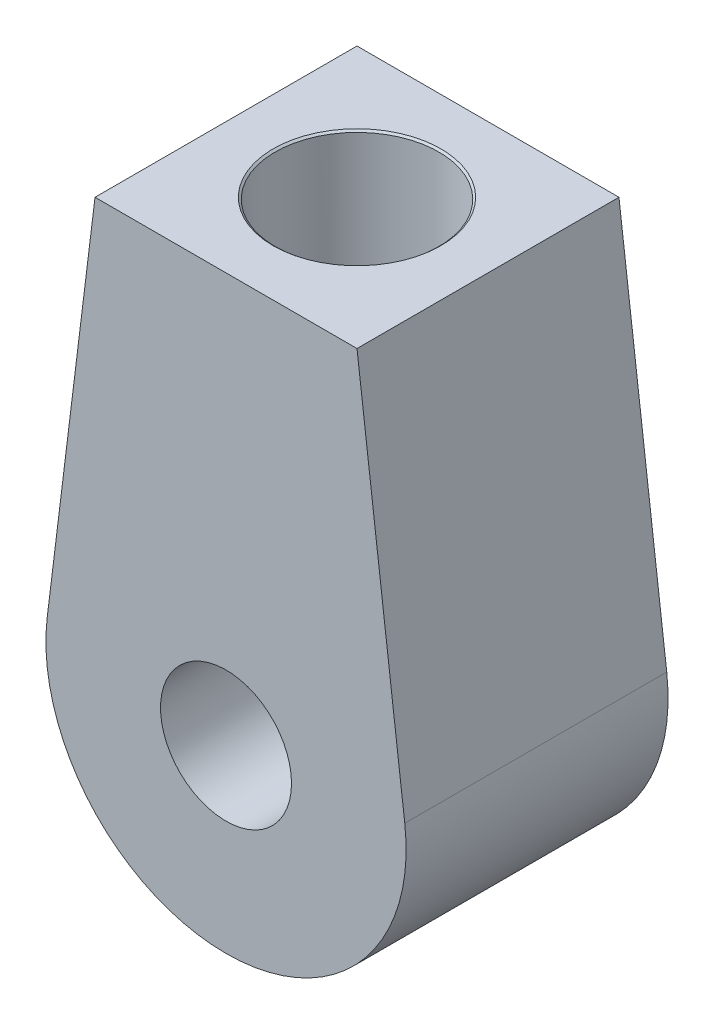
ISO-10303-21;
HEADER;
FILE_DESCRIPTION(('STEP AP214'),'2;1');
FILE_NAME('part.step','',(''),(''),'','','');
FILE_SCHEMA(('AUTOMOTIVE_DESIGN { 1 0 10303 214 1 1 1 1 }'));
ENDSEC;
DATA;
#1=APPLICATION_CONTEXT('core data for automotive mechanical design processes');
#2=APPLICATION_PROTOCOL_DEFINITION('international standard','automotive_design',2000,#1);
#3=PRODUCT_CONTEXT('',#1,'mechanical');
#4=PRODUCT('Part','Part','',(#3));
#5=PRODUCT_RELATED_PRODUCT_CATEGORY('part','',(#4));
#6=PRODUCT_DEFINITION_FORMATION('','',#4);
#7=PRODUCT_DEFINITION_CONTEXT('part definition',#1,'design');
#8=PRODUCT_DEFINITION('design','',#6,#7);
#9=PRODUCT_DEFINITION_SHAPE('','',#8);
#10=(LENGTH_UNIT() NAMED_UNIT(*) SI_UNIT(.MILLI.,.METRE.));
#11=(NAMED_UNIT(*) PLANE_ANGLE_UNIT() SI_UNIT($,.RADIAN.));
#12=(NAMED_UNIT(*) SI_UNIT($,.STERADIAN.) SOLID_ANGLE_UNIT());
#13=UNCERTAINTY_MEASURE_WITH_UNIT(LENGTH_MEASURE(1.E-05),#10,'distance_accuracy_value','');
#14=(GEOMETRIC_REPRESENTATION_CONTEXT(3) GLOBAL_UNCERTAINTY_ASSIGNED_CONTEXT((#13)) GLOBAL_UNIT_ASSIGNED_CONTEXT((#10,
#11,#12)) REPRESENTATION_CONTEXT('',''));
#15=CARTESIAN_POINT('',(0.,0.,0.));
#16=DIRECTION('',(0.,0.,1.));
#17=DIRECTION('',(1.,0.,0.));
#18=AXIS2_PLACEMENT_3D('',#15,#16,#17);
#19=CARTESIAN_POINT('',(-21.8345614174083,2.69294034642938,32.));
#20=DIRECTION('',(0.992480064427647,-0.122406379383154,0.));
#21=DIRECTION('',(0.122406379383154,0.992480064427648,0.));
#22=AXIS2_PLACEMENT_3D('',#19,#20,#21);
#23=PLANE('',#22);
#24=DIRECTION('',(-0.122406379383154,-0.992480064427648,0.));
#25=VECTOR('',#24,1.);
#26=CARTESIAN_POINT('',(-21.8345614174083,2.69294034642938,0.));
#27=LINE('',#26,#25);
#28=CARTESIAN_POINT('',(-16.,50.,0.));
#29=VERTEX_POINT('',#28);
#30=CARTESIAN_POINT('',(-21.8345614174083,2.69294034642938,0.));
#31=VERTEX_POINT('',#30);
#32=EDGE_CURVE('E192',#29,#31,#27,.T.);
#33=ORIENTED_EDGE('',*,*,#32,.T.);
#34=DIRECTION('',(0.,0.,-1.));
#35=VECTOR('',#34,1.);
#36=CARTESIAN_POINT('',(-21.8345614174083,2.69294034642938,32.));
#37=LINE('',#36,#35);
#38=CARTESIAN_POINT('',(-21.8345614174083,2.69294034642938,32.));
#39=VERTEX_POINT('',#38);
#40=EDGE_CURVE('E122',#39,#31,#37,.T.);
#41=ORIENTED_EDGE('',*,*,#40,.F.);
#42=DIRECTION('',(-0.122406379383154,-0.992480064427648,0.));
#43=VECTOR('',#42,1.);
#44=CARTESIAN_POINT('',(-21.8345614174083,2.69294034642938,32.));
#45=LINE('',#44,#43);
#46=CARTESIAN_POINT('',(-16.,50.,32.));
#47=VERTEX_POINT('',#46);
#48=EDGE_CURVE('E178',#47,#39,#45,.T.);
#49=ORIENTED_EDGE('',*,*,#48,.F.);
#50=DIRECTION('',(0.,0.,-1.));
#51=VECTOR('',#50,1.);
#52=CARTESIAN_POINT('',(-16.,50.,32.));
#53=LINE('',#52,#51);
#54=EDGE_CURVE('E69',#47,#29,#53,.T.);
#55=ORIENTED_EDGE('',*,*,#54,.T.);
#56=EDGE_LOOP('',(#33,#41,#49,#55));
#57=FACE_BOUND('',#56,.T.);
#58=ADVANCED_FACE('F41',(#57),#23,.F.);
#59=CARTESIAN_POINT('',(0.,0.,32.));
#60=DIRECTION('',(0.,0.,-1.));
#61=DIRECTION('',(-1.,0.,0.));
#62=AXIS2_PLACEMENT_3D('',#59,#60,#61);
#63=CYLINDRICAL_SURFACE('',#62,22.);
#64=CARTESIAN_POINT('',(0.,0.,0.));
#65=DIRECTION('',(0.,0.,1.));
#66=DIRECTION('',(1.,0.,0.));
#67=AXIS2_PLACEMENT_3D('',#64,#65,#66);
#68=CIRCLE('',#67,22.);
#69=CARTESIAN_POINT('',(21.8345614174083,2.69294034642938,0.));
#70=VERTEX_POINT('',#69);
#71=EDGE_CURVE('E194',#31,#70,#68,.T.);
#72=ORIENTED_EDGE('',*,*,#71,.T.);
#73=DIRECTION('',(0.,0.,-1.));
#74=VECTOR('',#73,1.);
#75=CARTESIAN_POINT('',(21.8345614174083,2.69294034642938,32.));
#76=LINE('',#75,#74);
#77=CARTESIAN_POINT('',(21.8345614174083,2.69294034642938,32.));
#78=VERTEX_POINT('',#77);
#79=EDGE_CURVE('E124',#78,#70,#76,.T.);
#80=ORIENTED_EDGE('',*,*,#79,.F.);
#81=CARTESIAN_POINT('',(0.,0.,32.));
#82=DIRECTION('',(0.,0.,1.));
#83=DIRECTION('',(1.,0.,0.));
#84=AXIS2_PLACEMENT_3D('',#81,#82,#83);
#85=CIRCLE('',#84,22.);
#86=EDGE_CURVE('E92',#39,#78,#85,.T.);
#87=ORIENTED_EDGE('',*,*,#86,.F.);
#88=ORIENTED_EDGE('',*,*,#40,.T.);
#89=EDGE_LOOP('',(#72,#80,#87,#88));
#90=FACE_BOUND('',#89,.T.);
#91=ADVANCED_FACE('F139',(#90),#63,.T.);
#92=CARTESIAN_POINT('',(21.8345614174083,2.69294034642937,32.));
#93=DIRECTION('',(0.992480064427648,0.122406379383153,0.));
#94=DIRECTION('',(-0.122406379383153,0.992480064427648,0.));
#95=AXIS2_PLACEMENT_3D('',#92,#93,#94);
#96=PLANE('',#95);
#97=DIRECTION('',(0.122406379383153,-0.992480064427648,0.));
#98=VECTOR('',#97,1.);
#99=CARTESIAN_POINT('',(21.8345614174083,2.69294034642937,0.));
#100=LINE('',#99,#98);
#101=CARTESIAN_POINT('',(16.,50.,0.));
#102=VERTEX_POINT('',#101);
#103=EDGE_CURVE('E198',#102,#70,#100,.T.);
#104=ORIENTED_EDGE('',*,*,#103,.F.);
#105=DIRECTION('',(0.,0.,-1.));
#106=VECTOR('',#105,1.);
#107=CARTESIAN_POINT('',(16.,50.,32.));
#108=LINE('',#107,#106);
#109=CARTESIAN_POINT('',(16.,50.,32.));
#110=VERTEX_POINT('',#109);
#111=EDGE_CURVE('E205',#110,#102,#108,.T.);
#112=ORIENTED_EDGE('',*,*,#111,.F.);
#113=DIRECTION('',(0.122406379383153,-0.992480064427648,0.));
#114=VECTOR('',#113,1.);
#115=CARTESIAN_POINT('',(21.8345614174083,2.69294034642937,32.));
#116=LINE('',#115,#114);
#117=EDGE_CURVE('E184',#110,#78,#116,.T.);
#118=ORIENTED_EDGE('',*,*,#117,.T.);
#119=ORIENTED_EDGE('',*,*,#79,.T.);
#120=EDGE_LOOP('',(#104,#112,#118,#119));
#121=FACE_BOUND('',#120,.T.);
#122=ADVANCED_FACE('F135',(#121),#96,.T.);
#123=CARTESIAN_POINT('',(0.,0.,32.));
#124=DIRECTION('',(0.,0.,-1.));
#125=DIRECTION('',(-1.,0.,0.));
#126=AXIS2_PLACEMENT_3D('',#123,#124,#125);
#127=CYLINDRICAL_SURFACE('',#126,8.);
#128=CARTESIAN_POINT('',(-8.,0.,10.));
#129=CARTESIAN_POINT('',(-8.00003518415619,0.151765783872228,10.000096854172));
#130=CARTESIAN_POINT('',(-7.99568301716214,0.30347310592064,9.99424436906945));
#131=CARTESIAN_POINT('',(-7.97848711233773,0.605311390024207,9.97139282513825));
#132=CARTESIAN_POINT('',(-7.96565778024779,0.755444588153614,9.95441267659789));
#133=CARTESIAN_POINT('',(-7.93201421856831,1.05121742892243,9.91034828500088));
#134=CARTESIAN_POINT('',(-7.91130847606391,1.19689027990274,9.88340145355975));
#135=CARTESIAN_POINT('',(-7.8623174610529,1.48503529687356,9.82055345855249));
#136=CARTESIAN_POINT('',(-7.83402843881417,1.62750584153131,9.78464786572442));
#137=CARTESIAN_POINT('',(-7.75894895631004,1.95881548521018,9.69100069433413));
#138=CARTESIAN_POINT('',(-7.70915840870956,2.14606620195669,9.6300387199926));
#139=CARTESIAN_POINT('',(-7.59749705485645,2.51293568124661,9.49726542647682));
#140=CARTESIAN_POINT('',(-7.53562203235276,2.69255175336717,9.42545032264953));
#141=CARTESIAN_POINT('',(-7.40017333549249,3.04521945414639,9.27334607877028));
#142=CARTESIAN_POINT('',(-7.32652140630302,3.21821683590856,9.19300155583507));
#143=CARTESIAN_POINT('',(-7.16846475696732,3.55639578231927,9.02674532132144));
#144=CARTESIAN_POINT('',(-7.08406004677426,3.72157735420221,8.94083361489623));
#145=CARTESIAN_POINT('',(-6.87272079550368,4.10227576591328,8.73400401947955));
#146=CARTESIAN_POINT('',(-6.74139999426485,4.31455990810847,8.61159688417738));
#147=CARTESIAN_POINT('',(-6.46024051292068,4.72516840260982,8.36453250968607));
#148=CARTESIAN_POINT('',(-6.31039531279453,4.92348780098436,8.2398744915134));
#149=CARTESIAN_POINT('',(-5.99279006154972,5.30547255162123,7.99206824857548));
#150=CARTESIAN_POINT('',(-5.82506400330904,5.48916458943401,7.86891763821471));
#151=CARTESIAN_POINT('',(-5.47166215392619,5.84150079918387,7.62702291754927));
#152=CARTESIAN_POINT('',(-5.28599236120471,6.01014996380691,7.50827735292303));
#153=CARTESIAN_POINT('',(-4.93525225938992,6.2995466919818,7.30079089860348));
#154=CARTESIAN_POINT('',(-4.77333113203328,6.42318519336549,7.21074800222999));
#155=CARTESIAN_POINT('',(-4.43827172586376,6.65910714375157,7.03688954107223));
#156=CARTESIAN_POINT('',(-4.26513562327791,6.77139278497195,6.95307277486531));
#157=CARTESIAN_POINT('',(-3.90819731115372,6.98348376083257,6.7932528339555));
#158=CARTESIAN_POINT('',(-3.72440596820847,7.08330149392986,6.71724191048984));
#159=CARTESIAN_POINT('',(-3.34664951394808,7.269404675154,6.57446649524366));
#160=CARTESIAN_POINT('',(-3.15268609866635,7.35569236969008,6.50770046873701));
#161=CARTESIAN_POINT('',(-2.78768776918432,7.50072541578791,6.39483677661395));
#162=CARTESIAN_POINT('',(-2.61801740950939,7.56166820428915,6.34714277384153));
#163=CARTESIAN_POINT('',(-2.27300673897084,7.67243442054968,6.26012965150418));
#164=CARTESIAN_POINT('',(-2.09766751588598,7.72225996722958,6.22080893607529));
#165=CARTESIAN_POINT('',(-1.7423411814074,7.8101040906857,6.15129425297338));
#166=CARTESIAN_POINT('',(-1.56235578100039,7.84812694854949,6.12109697614042));
#167=CARTESIAN_POINT('',(-1.19884884793697,7.91181432662965,6.0704263283358));
#168=CARTESIAN_POINT('',(-1.01532727306399,7.93747869920916,6.04995307352923));
#169=CARTESIAN_POINT('',(-0.645442355310554,7.97609552694194,6.01912008784497));
#170=CARTESIAN_POINT('',(-0.459071272708221,7.98900282986468,6.00879628048844));
#171=CARTESIAN_POINT('',(-0.0855945965198838,8.00172382938683,5.99862161786953));
#172=CARTESIAN_POINT('',(0.10151099848788,8.00153750062905,5.99877078288916));
#173=CARTESIAN_POINT('',(0.47494997983515,7.98807452538632,6.00953862466641));
#174=CARTESIAN_POINT('',(0.661283344469894,7.9747975134392,6.02015759371719));
#175=CARTESIAN_POINT('',(1.03170206758589,7.93538163057374,6.05162621931327));
#176=CARTESIAN_POINT('',(1.21578747786819,7.90924305660796,6.07247563965406));
#177=CARTESIAN_POINT('',(1.57035136569258,7.8463125528884,6.12253682575616));
#178=CARTESIAN_POINT('',(1.74102236622705,7.8101835821147,6.15122720358058));
#179=CARTESIAN_POINT('',(2.07820610240954,7.72730314871057,6.21682195318971));
#180=CARTESIAN_POINT('',(2.24471740468304,7.6805480790188,6.25372911409922));
#181=CARTESIAN_POINT('',(2.57265337699964,7.5770054193702,6.33511587763655));
#182=CARTESIAN_POINT('',(2.73407889593779,7.52021951427983,6.3795942084992));
#183=CARTESIAN_POINT('',(3.05122467601329,7.39722874621515,6.47542570243268));
#184=CARTESIAN_POINT('',(3.20694282253196,7.33102043566655,6.5267813814563));
#185=CARTESIAN_POINT('',(3.69396967375234,7.10564752564744,6.70051426420302));
#186=CARTESIAN_POINT('',(4.01352565933271,6.92968650116012,6.83463161582271));
#187=CARTESIAN_POINT('',(4.61897403100535,6.54176291196431,7.12430551985744));
#188=CARTESIAN_POINT('',(4.90485554933719,6.32978877835678,7.27986895860463));
#189=CARTESIAN_POINT('',(5.3351068398844,5.9650352696975,7.53995010807596));
#190=CARTESIAN_POINT('',(5.49061646582071,5.82214265659304,7.64022935328142));
#191=CARTESIAN_POINT('',(5.78887300220488,5.52568168737762,7.84392621336973));
#192=CARTESIAN_POINT('',(5.93162128734723,5.37211448434501,7.94734348860195));
#193=CARTESIAN_POINT('',(6.20458465993868,5.05441444466422,8.15572267513926));
#194=CARTESIAN_POINT('',(6.33476845245288,4.89025684303487,8.2606877289538));
#195=CARTESIAN_POINT('',(6.58206795781788,4.55195355242555,8.46988735848741));
#196=CARTESIAN_POINT('',(6.69918497819807,4.37780886545048,8.5741220063147));
#197=CARTESIAN_POINT('',(6.90962532089884,4.03650511397287,8.76980466284184));
#198=CARTESIAN_POINT('',(7.00415157295811,3.870245974404,8.86152885596269));
#199=CARTESIAN_POINT('',(7.18191416172241,3.52945259895588,9.04040251795251));
#200=CARTESIAN_POINT('',(7.26515278162993,3.35492004624695,9.12755290979307));
#201=CARTESIAN_POINT('',(7.41932541966022,2.9985122080723,9.29429918787117));
#202=CARTESIAN_POINT('',(7.49033255750238,2.81668918262712,9.3739385797172));
#203=CARTESIAN_POINT('',(7.61986804771234,2.44466403560352,9.52331980874378));
#204=CARTESIAN_POINT('',(7.67839821536092,2.25446313779137,9.59306308522082));
#205=CARTESIAN_POINT('',(7.77321772802353,1.89869333391319,9.70860052399917));
#206=CARTESIAN_POINT('',(7.81159147934962,1.73435301376588,9.75644968386134));
#207=CARTESIAN_POINT('',(7.87822912021012,1.40085504580776,9.8407470223142));
#208=CARTESIAN_POINT('',(7.90650035381239,1.23170099433526,9.87720348044821));
#209=CARTESIAN_POINT('',(7.95262661614723,0.886812152550988,9.93722747645968));
#210=CARTESIAN_POINT('',(7.97030886264618,0.711015490487897,9.96058084243755));
#211=CARTESIAN_POINT('',(7.98807956621915,0.445533946342427,9.98413170056095));
#212=CARTESIAN_POINT('',(7.99254444956147,0.356607500151852,9.99006903283161));
#213=CARTESIAN_POINT('',(7.99850624224261,0.178460509600567,9.99800781596778));
#214=CARTESIAN_POINT('',(8.00000248720756,0.0892399038817475,10.0000083857949));
#215=CARTESIAN_POINT('',(8.00000000000005,-1.01988353627275E-13,9.99999999999968));
#216=B_SPLINE_CURVE_WITH_KNOTS('',3,(#128,#129,#130,#131,#132,#133,#134,#135,#136,#137,#138,
#139,#140,#141,#142,#143,#144,#145,#146,#147,#148,#149,#150,#151,#152,#153,#154,#155,#156,#157,
#158,#159,#160,#161,#162,#163,#164,#165,#166,#167,#168,#169,#170,#171,#172,#173,#174,#175,#176,
#177,#178,#179,#180,#181,#182,#183,#184,#185,#186,#187,#188,#189,#190,#191,#192,#193,#194,#195,
#196,#197,#198,#199,#200,#201,#202,#203,#204,#205,#206,#207,#208,#209,#210,#211,#212,#213,#214,
#215),.UNSPECIFIED.,.F.,.F.,(4,2,2,2,2,2,2,2,2,2,2,2,2,2,2,2,2,2,2,2,2,2,2,2,2,2,2,2,2,2,2,2,2,
2,2,2,2,2,2,2,2,2,2,4),(0.,0.455028773871634,0.909286272689605,1.35750113375535,
1.80593803539875,2.41433904521739,3.02295270546237,3.63579274485763,4.2486322169897,
5.08160930483717,5.91488041430752,6.74659474499211,7.57803199688832,8.24565046751402,
8.91313977494568,9.5799599353767,10.2466692653234,10.8055624323806,11.3643489845224,
11.9229326153529,12.481522918966,13.0420832856594,13.6026447379371,14.1632218402617,
14.7237860003801,15.2536038826881,15.7836018826097,16.3135109439567,16.8436143951966,
18.0050651995015,19.1668898177403,19.8677038774358,20.5684423518877,21.2708834274713,
21.9732541499751,22.6091179801846,23.2448529987567,23.8766447185808,24.5083444558741,
25.0339422784753,25.5591572344839,26.0927239124872,26.3603118377474,26.6279596417657),.UNSPECIFIED.);
#217=CARTESIAN_POINT('',(-8.,0.,10.));
#218=VERTEX_POINT('',#217);
#219=CARTESIAN_POINT('',(8.,0.,10.));
#220=VERTEX_POINT('',#219);
#221=EDGE_CURVE('E11',#218,#220,#216,.T.);
#222=ORIENTED_EDGE('',*,*,#221,.F.);
#223=DIRECTION('',(0.,0.,-1.));
#224=VECTOR('',#223,1.);
#225=CARTESIAN_POINT('',(-8.,0.,32.));
#226=LINE('',#225,#224);
#227=CARTESIAN_POINT('',(-8.,0.,22.));
#228=VERTEX_POINT('',#227);
#229=EDGE_CURVE('E52',#228,#218,#226,.T.);
#230=ORIENTED_EDGE('',*,*,#229,.F.);
#231=CARTESIAN_POINT('',(8.,0.,22.));
#232=CARTESIAN_POINT('',(8.00003518415619,0.151765783872227,21.9999031458279));
#233=CARTESIAN_POINT('',(7.99568301716214,0.303473105920638,22.0057556309305));
#234=CARTESIAN_POINT('',(7.97848711233774,0.605311390024205,22.0286071748617));
#235=CARTESIAN_POINT('',(7.96565778024779,0.755444588153612,22.0455873234021));
#236=CARTESIAN_POINT('',(7.93201421856831,1.05121742892242,22.0896517149991));
#237=CARTESIAN_POINT('',(7.91130847606391,1.19689027990273,22.1165985464402));
#238=CARTESIAN_POINT('',(7.8623174610529,1.48503529687355,22.1794465414475));
#239=CARTESIAN_POINT('',(7.83402843881417,1.62750584153131,22.2153521342755));
#240=CARTESIAN_POINT('',(7.75894895631005,1.95881548521017,22.3089993056658));
#241=CARTESIAN_POINT('',(7.70915840870956,2.14606620195668,22.3699612800074));
#242=CARTESIAN_POINT('',(7.59749705485645,2.5129356812466,22.5027345735232));
#243=CARTESIAN_POINT('',(7.53562203235277,2.69255175336716,22.5745496773504));
#244=CARTESIAN_POINT('',(7.40017333549249,3.04521945414638,22.7266539212297));
#245=CARTESIAN_POINT('',(7.32652140630303,3.21821683590855,22.8069984441649));
#246=CARTESIAN_POINT('',(7.16846475696733,3.55639578231926,22.9732546786785));
#247=CARTESIAN_POINT('',(7.08406004677427,3.7215773542022,23.0591663851037));
#248=CARTESIAN_POINT('',(6.87272079550369,4.10227576591326,23.2659959805204));
#249=CARTESIAN_POINT('',(6.74139999426486,4.31455990810846,23.3884031158226));
#250=CARTESIAN_POINT('',(6.46024051292069,4.72516840260981,23.6354674903139));
#251=CARTESIAN_POINT('',(6.31039531279454,4.92348780098435,23.7601255084866));
#252=CARTESIAN_POINT('',(5.99279006154973,5.30547255162122,24.0079317514245));
#253=CARTESIAN_POINT('',(5.82506400330905,5.48916458943401,24.1310823617853));
#254=CARTESIAN_POINT('',(5.4716621539262,5.84150079918386,24.3729770824507));
#255=CARTESIAN_POINT('',(5.28599236120472,6.0101499638069,24.491722647077));
#256=CARTESIAN_POINT('',(4.93525225938993,6.29954669198179,24.6992091013965));
#257=CARTESIAN_POINT('',(4.77333113203329,6.42318519336549,24.78925199777));
#258=CARTESIAN_POINT('',(4.43827172586377,6.65910714375156,24.9631104589278));
#259=CARTESIAN_POINT('',(4.26513562327792,6.77139278497195,25.0469272251347));
#260=CARTESIAN_POINT('',(3.90819731115373,6.98348376083256,25.2067471660445));
#261=CARTESIAN_POINT('',(3.72440596820848,7.08330149392986,25.2827580895101));
#262=CARTESIAN_POINT('',(3.34664951394809,7.26940467515399,25.4255335047563));
#263=CARTESIAN_POINT('',(3.15268609866636,7.35569236969007,25.492299531263));
#264=CARTESIAN_POINT('',(2.78768776918433,7.5007254157879,25.605163223386));
#265=CARTESIAN_POINT('',(2.61801740950939,7.56166820428914,25.6528572261585));
#266=CARTESIAN_POINT('',(2.27300673897085,7.67243442054967,25.7398703484958));
#267=CARTESIAN_POINT('',(2.09766751588599,7.72225996722957,25.7791910639247));
#268=CARTESIAN_POINT('',(1.74234118140741,7.8101040906857,25.8487057470266));
#269=CARTESIAN_POINT('',(1.56235578100039,7.84812694854949,25.8789030238596));
#270=CARTESIAN_POINT('',(1.19884884793698,7.91181432662965,25.9295736716642));
#271=CARTESIAN_POINT('',(1.01532727306399,7.93747869920916,25.9500469264708));
#272=CARTESIAN_POINT('',(0.645442355310562,7.97609552694194,25.980879912155));
#273=CARTESIAN_POINT('',(0.459071272708229,7.98900282986468,25.9912037195116));
#274=CARTESIAN_POINT('',(0.0855945965198925,8.00172382938683,26.0013783821305));
#275=CARTESIAN_POINT('',(-0.101510998487871,8.00153750062905,26.0012292171108));
#276=CARTESIAN_POINT('',(-0.474949979835142,7.98807452538632,25.9904613753336));
#277=CARTESIAN_POINT('',(-0.661283344469887,7.9747975134392,25.9798424062828));
#278=CARTESIAN_POINT('',(-1.03170206758588,7.93538163057374,25.9483737806867));
#279=CARTESIAN_POINT('',(-1.21578747786818,7.90924305660796,25.9275243603459));
#280=CARTESIAN_POINT('',(-1.57035136569258,7.8463125528884,25.8774631742438));
#281=CARTESIAN_POINT('',(-1.74102236622704,7.8101835821147,25.8487727964194));
#282=CARTESIAN_POINT('',(-2.07820610240953,7.72730314871057,25.7831780468103));
#283=CARTESIAN_POINT('',(-2.24471740468304,7.68054807901881,25.7462708859008));
#284=CARTESIAN_POINT('',(-2.57265337699963,7.57700541937021,25.6648841223635));
#285=CARTESIAN_POINT('',(-2.73407889593779,7.52021951427984,25.6204057915008));
#286=CARTESIAN_POINT('',(-3.05122467601328,7.39722874621515,25.5245742975673));
#287=CARTESIAN_POINT('',(-3.20694282253195,7.33102043566655,25.4732186185437));
#288=CARTESIAN_POINT('',(-3.69396967375234,7.10564752564745,25.299485735797));
#289=CARTESIAN_POINT('',(-4.01352565933271,6.92968650116012,25.1653683841773));
#290=CARTESIAN_POINT('',(-4.61897403100534,6.54176291196432,24.8756944801426));
#291=CARTESIAN_POINT('',(-4.90485554933719,6.32978877835679,24.7201310413954));
#292=CARTESIAN_POINT('',(-5.3351068398844,5.9650352696975,24.4600498919241));
#293=CARTESIAN_POINT('',(-5.49061646582071,5.82214265659304,24.3597706467186));
#294=CARTESIAN_POINT('',(-5.78887300220488,5.52568168737763,24.1560737866303));
#295=CARTESIAN_POINT('',(-5.93162128734722,5.37211448434502,24.0526565113981));
#296=CARTESIAN_POINT('',(-6.20458465993868,5.05441444466423,23.8442773248608));
#297=CARTESIAN_POINT('',(-6.33476845245287,4.89025684303488,23.7393122710462));
#298=CARTESIAN_POINT('',(-6.58206795781787,4.55195355242556,23.5301126415126));
#299=CARTESIAN_POINT('',(-6.69918497819807,4.37780886545049,23.4258779936853));
#300=CARTESIAN_POINT('',(-6.90962532089884,4.03650511397288,23.2301953371582));
#301=CARTESIAN_POINT('',(-7.00415157295811,3.87024597440401,23.1384711440373));
#302=CARTESIAN_POINT('',(-7.18191416172241,3.52945259895589,22.9595974820475));
#303=CARTESIAN_POINT('',(-7.26515278162993,3.35492004624696,22.872447090207));
#304=CARTESIAN_POINT('',(-7.41932541966021,2.99851220807231,22.7057008121289));
#305=CARTESIAN_POINT('',(-7.49033255750238,2.81668918262713,22.6260614202828));
#306=CARTESIAN_POINT('',(-7.61986804771234,2.44466403560353,22.4766801912562));
#307=CARTESIAN_POINT('',(-7.67839821536092,2.25446313779138,22.4069369147792));
#308=CARTESIAN_POINT('',(-7.77321772802353,1.89869333391319,22.2913994760009));
#309=CARTESIAN_POINT('',(-7.81159147934962,1.73435301376588,22.2435503161387));
#310=CARTESIAN_POINT('',(-7.87822912021012,1.40085504580776,22.1592529776858));
#311=CARTESIAN_POINT('',(-7.90650035381238,1.23170099433527,22.1227965195518));
#312=CARTESIAN_POINT('',(-7.95262661614723,0.886812152550992,22.0627725235403));
#313=CARTESIAN_POINT('',(-7.97030886264618,0.711015490487901,22.0394191575625));
#314=CARTESIAN_POINT('',(-7.98807956621915,0.44553394634243,22.0158682994391));
#315=CARTESIAN_POINT('',(-7.99254444956147,0.356607500151854,22.0099309671684));
#316=CARTESIAN_POINT('',(-7.99850624224261,0.178460509600569,22.0019921840322));
#317=CARTESIAN_POINT('',(-8.00000248720756,0.089239903881749,21.9999916142052));
#318=CARTESIAN_POINT('',(-8.00000000000005,-1.00478074753769E-13,22.0000000000003));
#319=B_SPLINE_CURVE_WITH_KNOTS('',3,(#231,#232,#233,#234,#235,#236,#237,#238,#239,#240,#241,
#242,#243,#244,#245,#246,#247,#248,#249,#250,#251,#252,#253,#254,#255,#256,#257,#258,#259,#260,
#261,#262,#263,#264,#265,#266,#267,#268,#269,#270,#271,#272,#273,#274,#275,#276,#277,#278,#279,
#280,#281,#282,#283,#284,#285,#286,#287,#288,#289,#290,#291,#292,#293,#294,#295,#296,#297,#298,
#299,#300,#301,#302,#303,#304,#305,#306,#307,#308,#309,#310,#311,#312,#313,#314,#315,#316,#317,
#318),.UNSPECIFIED.,.F.,.F.,(4,2,2,2,2,2,2,2,2,2,2,2,2,2,2,2,2,2,2,2,2,2,2,2,2,2,2,2,2,2,2,2,2,
2,2,2,2,2,2,2,2,2,2,4),(0.,0.455028773871632,0.909286272689601,1.35750113375535,
1.80593803539874,2.41433904521738,3.02295270546236,3.63579274485762,4.24863221698969,
5.08160930483715,5.91488041430751,6.7465947449921,7.57803199688831,8.24565046751402,
8.91313977494568,9.5799599353767,10.2466692653234,10.8055624323806,11.3643489845224,
11.9229326153529,12.481522918966,13.0420832856594,13.6026447379371,14.1632218402617,
14.7237860003801,15.2536038826881,15.7836018826097,16.3135109439567,16.8436143951966,
18.0050651995015,19.1668898177403,19.8677038774358,20.5684423518877,21.2708834274713,
21.973254149975,22.6091179801845,23.2448529987567,23.8766447185808,24.5083444558741,
25.0339422784753,25.5591572344839,26.0927239124872,26.3603118377474,26.6279596417657),.UNSPECIFIED.);
#320=CARTESIAN_POINT('',(8.,0.,22.));
#321=VERTEX_POINT('',#320);
#322=EDGE_CURVE('E114',#321,#228,#319,.T.);
#323=ORIENTED_EDGE('',*,*,#322,.F.);
#324=DIRECTION('',(0.,0.,-1.));
#325=VECTOR('',#324,1.);
#326=CARTESIAN_POINT('',(8.,0.,32.));
#327=LINE('',#326,#325);
#328=EDGE_CURVE('E106',#220,#321,#327,.F.);
#329=ORIENTED_EDGE('',*,*,#328,.F.);
#330=EDGE_LOOP('',(#222,#230,#323,#329));
#331=FACE_BOUND('',#330,.T.);
#332=CARTESIAN_POINT('',(0.,0.,32.));
#333=DIRECTION('',(0.,0.,1.));
#334=DIRECTION('',(1.,0.,0.));
#335=AXIS2_PLACEMENT_3D('',#332,#333,#334);
#336=CIRCLE('',#335,8.);
#337=CARTESIAN_POINT('',(8.,0.,32.));
#338=VERTEX_POINT('',#337);
#339=EDGE_CURVE('E180',#338,#338,#336,.T.);
#340=ORIENTED_EDGE('',*,*,#339,.T.);
#341=EDGE_LOOP('',(#340));
#342=FACE_BOUND('',#341,.T.);
#343=CARTESIAN_POINT('',(0.,0.,0.));
#344=DIRECTION('',(0.,0.,1.));
#345=DIRECTION('',(1.,0.,0.));
#346=AXIS2_PLACEMENT_3D('',#343,#344,#345);
#347=CIRCLE('',#346,8.);
#348=CARTESIAN_POINT('',(8.,0.,0.));
#349=VERTEX_POINT('',#348);
#350=EDGE_CURVE('E118',#349,#349,#347,.T.);
#351=ORIENTED_EDGE('',*,*,#350,.F.);
#352=EDGE_LOOP('',(#351));
#353=FACE_BOUND('',#352,.T.);
#354=ADVANCED_FACE('F120',(#331,#342,#353),#127,.F.);
#355=CARTESIAN_POINT('',(0.,50.,32.));
#356=DIRECTION('',(0.,1.,0.));
#357=DIRECTION('',(-1.,0.,0.));
#358=AXIS2_PLACEMENT_3D('',#355,#356,#357);
#359=PLANE('',#358);
#360=CARTESIAN_POINT('',(0.,50.,16.));
#361=DIRECTION('',(0.,1.,0.));
#362=DIRECTION('',(0.,0.,1.));
#363=AXIS2_PLACEMENT_3D('',#360,#361,#362);
#364=CIRCLE('',#363,10.25);
#365=CARTESIAN_POINT('',(0.,50.,26.25));
#366=VERTEX_POINT('',#365);
#367=EDGE_CURVE('E172',#366,#366,#364,.T.);
#368=ORIENTED_EDGE('',*,*,#367,.F.);
#369=EDGE_LOOP('',(#368));
#370=FACE_BOUND('',#369,.T.);
#371=DIRECTION('',(1.,0.,0.));
#372=VECTOR('',#371,1.);
#373=CARTESIAN_POINT('',(0.,50.,0.));
#374=LINE('',#373,#372);
#375=EDGE_CURVE('E182',#29,#102,#374,.T.);
#376=ORIENTED_EDGE('',*,*,#375,.F.);
#377=ORIENTED_EDGE('',*,*,#54,.F.);
#378=DIRECTION('',(1.,0.,0.));
#379=VECTOR('',#378,1.);
#380=CARTESIAN_POINT('',(0.,50.,32.));
#381=LINE('',#380,#379);
#382=EDGE_CURVE('E189',#47,#110,#381,.T.);
#383=ORIENTED_EDGE('',*,*,#382,.T.);
#384=ORIENTED_EDGE('',*,*,#111,.T.);
#385=EDGE_LOOP('',(#376,#377,#383,#384));
#386=FACE_BOUND('',#385,.T.);
#387=ADVANCED_FACE('F132',(#370,#386),#359,.T.);
#388=CARTESIAN_POINT('',(0.,0.,32.));
#389=DIRECTION('',(0.,0.,1.));
#390=DIRECTION('',(1.,0.,0.));
#391=AXIS2_PLACEMENT_3D('',#388,#389,#390);
#392=PLANE('',#391);
#393=ORIENTED_EDGE('',*,*,#339,.F.);
#394=EDGE_LOOP('',(#393));
#395=FACE_BOUND('',#394,.T.);
#396=ORIENTED_EDGE('',*,*,#48,.T.);
#397=ORIENTED_EDGE('',*,*,#86,.T.);
#398=ORIENTED_EDGE('',*,*,#117,.F.);
#399=ORIENTED_EDGE('',*,*,#382,.F.);
#400=EDGE_LOOP('',(#396,#397,#398,#399));
#401=FACE_BOUND('',#400,.T.);
#402=ADVANCED_FACE('F148',(#395,#401),#392,.T.);
#403=CARTESIAN_POINT('',(0.,0.,0.));
#404=DIRECTION('',(0.,0.,1.));
#405=DIRECTION('',(1.,0.,0.));
#406=AXIS2_PLACEMENT_3D('',#403,#404,#405);
#407=PLANE('',#406);
#408=ORIENTED_EDGE('',*,*,#350,.T.);
#409=EDGE_LOOP('',(#408));
#410=FACE_BOUND('',#409,.T.);
#411=ORIENTED_EDGE('',*,*,#32,.F.);
#412=ORIENTED_EDGE('',*,*,#375,.T.);
#413=ORIENTED_EDGE('',*,*,#103,.T.);
#414=ORIENTED_EDGE('',*,*,#71,.F.);
#415=EDGE_LOOP('',(#411,#412,#413,#414));
#416=FACE_BOUND('',#415,.T.);
#417=ADVANCED_FACE('F146',(#410,#416),#407,.F.);
#418=CARTESIAN_POINT('',(0.,0.,16.));
#419=DIRECTION('',(0.,-1.,0.));
#420=DIRECTION('',(0.,0.,-1.));
#421=AXIS2_PLACEMENT_3D('',#418,#419,#420);
#422=PLANE('',#421);
#423=ORIENTED_EDGE('',*,*,#229,.T.);
#424=CARTESIAN_POINT('',(0.,0.,16.));
#425=DIRECTION('',(0.,1.,0.));
#426=DIRECTION('',(0.,0.,1.));
#427=AXIS2_PLACEMENT_3D('',#424,#425,#426);
#428=CIRCLE('',#427,9.99999999999999);
#429=EDGE_CURVE('E56',#218,#228,#428,.T.);
#430=ORIENTED_EDGE('',*,*,#429,.T.);
#431=EDGE_LOOP('',(#423,#430));
#432=FACE_BOUND('',#431,.T.);
#433=ADVANCED_FACE('F151',(#432),#422,.F.);
#434=ORIENTED_EDGE('',*,*,#328,.T.);
#435=EDGE_CURVE('E108',#321,#220,#428,.T.);
#436=ORIENTED_EDGE('',*,*,#435,.T.);
#437=EDGE_LOOP('',(#434,#436));
#438=FACE_BOUND('',#437,.T.);
#439=ADVANCED_FACE('F107',(#438),#422,.F.);
#440=CARTESIAN_POINT('',(0.,50.,16.));
#441=DIRECTION('',(0.,1.,0.));
#442=DIRECTION('',(0.,0.,1.));
#443=AXIS2_PLACEMENT_3D('',#440,#441,#442);
#444=CYLINDRICAL_SURFACE('',#443,9.99999999999999);
#445=CARTESIAN_POINT('',(0.,49.7902250922057,16.));
#446=DIRECTION('',(0.,1.,0.));
#447=DIRECTION('',(0.,0.,1.));
#448=AXIS2_PLACEMENT_3D('',#445,#446,#447);
#449=CIRCLE('',#448,9.99999999999999);
#450=CARTESIAN_POINT('',(0.,49.7902250922057,26.));
#451=VERTEX_POINT('',#450);
#452=EDGE_CURVE('E168',#451,#451,#449,.T.);
#453=ORIENTED_EDGE('',*,*,#452,.T.);
#454=EDGE_LOOP('',(#453));
#455=FACE_BOUND('',#454,.T.);
#456=ORIENTED_EDGE('',*,*,#221,.T.);
#457=ORIENTED_EDGE('',*,*,#435,.F.);
#458=ORIENTED_EDGE('',*,*,#322,.T.);
#459=ORIENTED_EDGE('',*,*,#429,.F.);
#460=EDGE_LOOP('',(#456,#457,#458,#459));
#461=FACE_BOUND('',#460,.T.);
#462=ADVANCED_FACE('F113',(#455,#461),#444,.F.);
#463=CARTESIAN_POINT('',(0.,50.,16.));
#464=DIRECTION('',(0.,1.,0.));
#465=DIRECTION('',(0.,0.,1.));
#466=AXIS2_PLACEMENT_3D('',#463,#464,#465);
#467=CONICAL_SURFACE('',#466,10.25,0.872664625997171);
#468=ORIENTED_EDGE('',*,*,#452,.F.);
#469=EDGE_LOOP('',(#468));
#470=FACE_BOUND('',#469,.T.);
#471=ORIENTED_EDGE('',*,*,#367,.T.);
#472=EDGE_LOOP('',(#471));
#473=FACE_BOUND('',#472,.T.);
#474=ADVANCED_FACE('F158',(#470,#473),#467,.F.);
#475=CLOSED_SHELL('',(#58,#91,#122,#354,#387,#402,#417,#433,#439,#462,#474));
#476=MANIFOLD_SOLID_BREP('B2',#475);
#477=ADVANCED_BREP_SHAPE_REPRESENTATION('',(#18,#476),#14);
#478=SHAPE_DEFINITION_REPRESENTATION(#9,#477);
ENDSEC;
END-ISO-10303-21;
